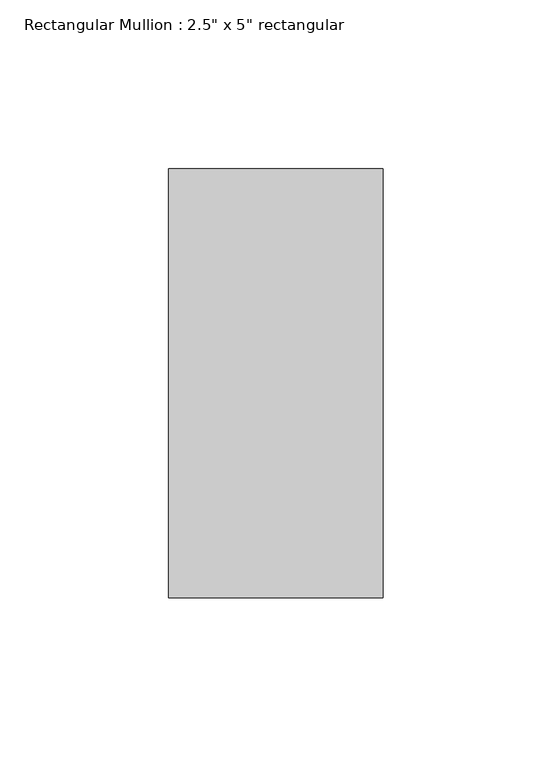
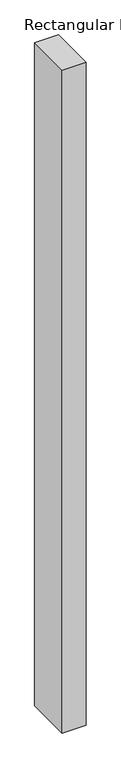
"""IFC4 building model written with IfcOpenShell, lengths in millimetres: member geometry."""

from ifc_helpers import new_model, si_unit, frame, origin, place, context, project, spatial, polyline, outline, extrude, source, transform, mapped, element, save


def member_719f051b(model_context):
    return source(origin(), model_context, "Body", "SweptSolid", [
        extrude(outline(polyline([(0.0, 63.5), (0.0, -63.5), (-63.5, -63.5), (-63.5, 63.5), (0.0, 63.5)])), frame((0.0, 0.0, -1868.0529055), z_axis=(0.0, 0.0, 1.0), x_axis=(1.0, 0.0, 0.0)), (0.0, 0.0, 1.0), 1868.0529055),
    ])


if __name__ == "__main__":
    model = new_model("IFC4")
    model_context = context("Model", 3, world=origin())
    ifc_project = project(units=[si_unit("LENGTHUNIT", "METRE", prefix="MILLI")], contexts=[model_context])
    site = spatial("IfcSite", under=ifc_project)
    building = spatial("IfcBuilding", under=site)
    placement = place(None, origin())
    member_shape = member_719f051b(model_context)
    element("IfcMember", 1, ObjectType="Rectangular Mullion : 2.5\" x 5\" rectangular", at=placement, inside=building, context=model_context, shape_type="MappedRepresentation", body=[
        mapped(member_shape, transform((0.0, 0.0, 0.0), x_axis=(1.0, 0.0, 0.0), y_axis=(0.0, 1.0, 0.0), z_axis=(0.0, 0.0, 1.0))),
    ])
    save(model, "model.ifc")

# Revit data of these elements
# Type "Rectangular Mullion : 2.5\" x 5\" rectangular"
#   built-in parameter 1007304 = 0.416667 (stored number, unit not read)
#   built-in parameter 1007301 = 0.104167 (stored number, unit not read)
#   built-in parameter 1007300 = 0.104167 (stored number, unit not read)
# Element 1 (IfcMember, "Rectangular Mullion : 2.5\" x 5\" rectangular")
#   Materials on its faces: "Aluminum"
# Materials
#   "Aluminum": class "Metal", colour RGB 247 247 247, transparency 0, Description = "Aluminum 6061", Cost = 0
